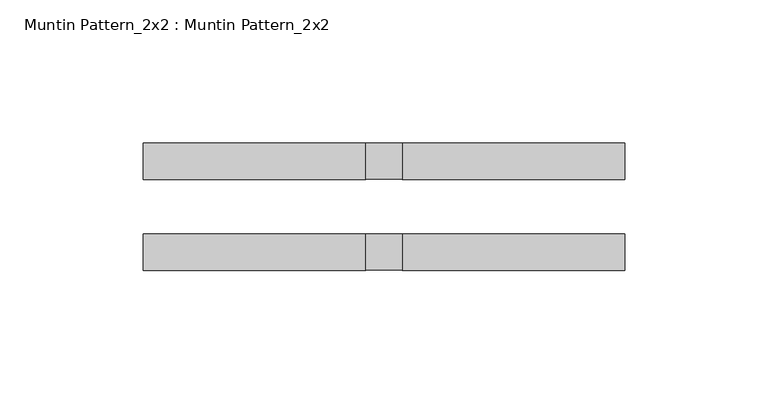
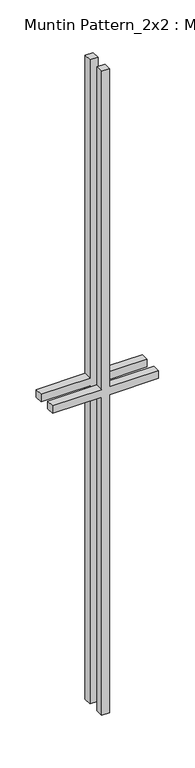
"""IFC4 building model written with IfcOpenShell, lengths in millimetres: proxy geometry, Muntin Pattern_2x2 : Muntin Pattern_2x2."""

from ifc_helpers import new_model, si_unit, frame, origin, place, context, project, spatial, polyline, outline, extrude, source, transform, mapped, element, save


def muntin_pattern_2x2_muntin_pattern_2x2_784a3213(model_context):
    return source(origin(), model_context, "Body", "SweptSolid", [
        extrude(outline(polyline([(546.1, -6.35), (546.1, -84.1375), (533.4, -84.1375), (533.4, -6.35), (0.0, -6.35), (0.0, 6.35), (533.4, 6.35), (533.4, 84.1375), (546.1, 84.1375), (546.1, 6.35), (1079.5, 6.35), (1079.5, -6.35), (546.1, -6.35)])), frame((0.0, -22.225, 0.0), z_axis=(0.0, 1.0, 0.0), x_axis=(0.0, 0.0, 1.0)), (0.0, 0.0, 1.0), 12.7),
        extrude(outline(polyline([(546.1, -6.35), (546.1, -84.1375), (533.4, -84.1375), (533.4, -6.35), (0.0, -6.35), (0.0, 6.35), (533.4, 6.35), (533.4, 84.1375), (546.1, 84.1375), (546.1, 6.35), (1079.5, 6.35), (1079.5, -6.35), (546.1, -6.35)])), frame((0.0, 9.525, 0.0), z_axis=(0.0, 1.0, 0.0), x_axis=(0.0, 0.0, 1.0)), (0.0, 0.0, 1.0), 12.7),
    ])


if __name__ == "__main__":
    model = new_model("IFC4")
    model_context = context("Model", 3, world=origin())
    ifc_project = project(units=[si_unit("LENGTHUNIT", "METRE", prefix="MILLI")], contexts=[model_context])
    site = spatial("IfcSite", under=ifc_project)
    building = spatial("IfcBuilding", under=site)
    placement = place(None, origin())
    muntin_pattern_2x2_muntin_pattern_2x2_shape = muntin_pattern_2x2_muntin_pattern_2x2_784a3213(model_context)
    element("IfcBuildingElementProxy", 1, Name="Muntin Pattern_2x2 : Muntin Pattern_2x2", ObjectType="Muntin Pattern_2x2 : Muntin Pattern_2x2", at=placement, inside=building, context=model_context, shape_type="MappedRepresentation", body=[
        mapped(muntin_pattern_2x2_muntin_pattern_2x2_shape, transform((0.0, 0.0, 0.0), x_axis=(1.0, 0.0, 0.0), y_axis=(0.0, 1.0, 0.0), z_axis=(0.0, 0.0, 1.0))),
    ])
    save(model, "model.ifc")

# Revit data of these elements
# Type "Muntin Pattern_2x2 : Muntin Pattern_2x2"
#   Width [instance default] = 4' - 0"
#   Thickness = 0' - 0 1/2"
#   Height [instance default] = 4' - 0"
#   Distance = 0' - 0 3/4"
#   Interior Material [instance default] = none
#   Exterior Material [instance default] = none
#   Default Elevation = 0
# Element 1 (IfcBuildingElementProxy, "Muntin Pattern_2x2 : Muntin Pattern_2x2")
#   Width = 0' - 6 5/8"
#   Height = 3' - 6 1/2"
#   Interior Material = Wood - Stained
#   Exterior Material = Clad - White
#   Materials on its faces: "Clad - White", "Wood - Stained"
# Materials
#   "Clad - White": class "Wood", colour RGB 242 242 238, transparency 0, Cost = 0
#   "Wood - Stained": class "Wood", colour RGB 224 178 126, transparency 0, Cost = 0
